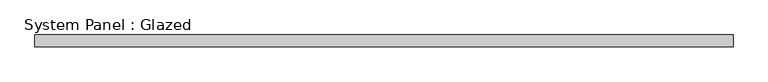
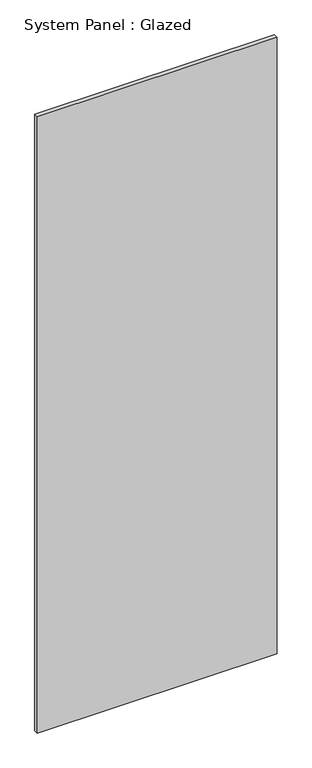
"""IFC4 building model written with IfcOpenShell, lengths in millimetres: plate geometry, System Panel : Glazed."""

from ifc_helpers import new_model, si_unit, origin, origin_with_axes, place, context, project, spatial, polyline, outline, extrude, source, transform, mapped, element, save


def system_panel_glazed_5123bacf(model_context):
    return source(origin(), model_context, "Body", "SweptSolid", [
        extrude(outline(polyline([(736.6, 24.5), (-736.6, 24.5), (-736.6, 49.5), (736.6, 49.5), (736.6, 24.5)])), origin_with_axes(), (0.0, 0.0, 1.0), 4000.0),
    ])


if __name__ == "__main__":
    model = new_model("IFC4")
    model_context = context("Model", 3, world=origin())
    ifc_project = project(units=[si_unit("LENGTHUNIT", "METRE", prefix="MILLI")], contexts=[model_context])
    site = spatial("IfcSite", under=ifc_project)
    building = spatial("IfcBuilding", under=site)
    placement = place(None, origin())
    system_panel_glazed_shape = system_panel_glazed_5123bacf(model_context)
    element("IfcPlate", 1, ObjectType="System Panel : Glazed", at=placement, inside=building, context=model_context, shape_type="MappedRepresentation", body=[
        mapped(system_panel_glazed_shape, transform((0.0, 0.0, 0.0), x_axis=(1.0, 0.0, 0.0), y_axis=(0.0, 1.0, 0.0), z_axis=(0.0, 0.0, 1.0))),
    ])
    save(model, "model.ifc")

# Revit data of these elements
# Type "System Panel : Glazed"
#   Keynote = "H11"
#   Construction Type Id = "GSP4R"
#   Analytic Construction = "1/8 in Pilkington single glazing"
#   Visual Light Transmittance = 0.9
#   Solar Heat Gain Coefficient = 0.86
#   Heat Transfer Coefficient (U) = 6.7069 W/(m²·K)
#   Define Thermal Properties by = 1
# Element 1 (IfcPlate, "System Panel : Glazed")
#   Materials on its faces: "Glass"
# Materials
#   "Glass": class "Glass", colour RGB 0 128 192, transparency 0.9, Description = "Soda Lime Glass", Cost = 0
